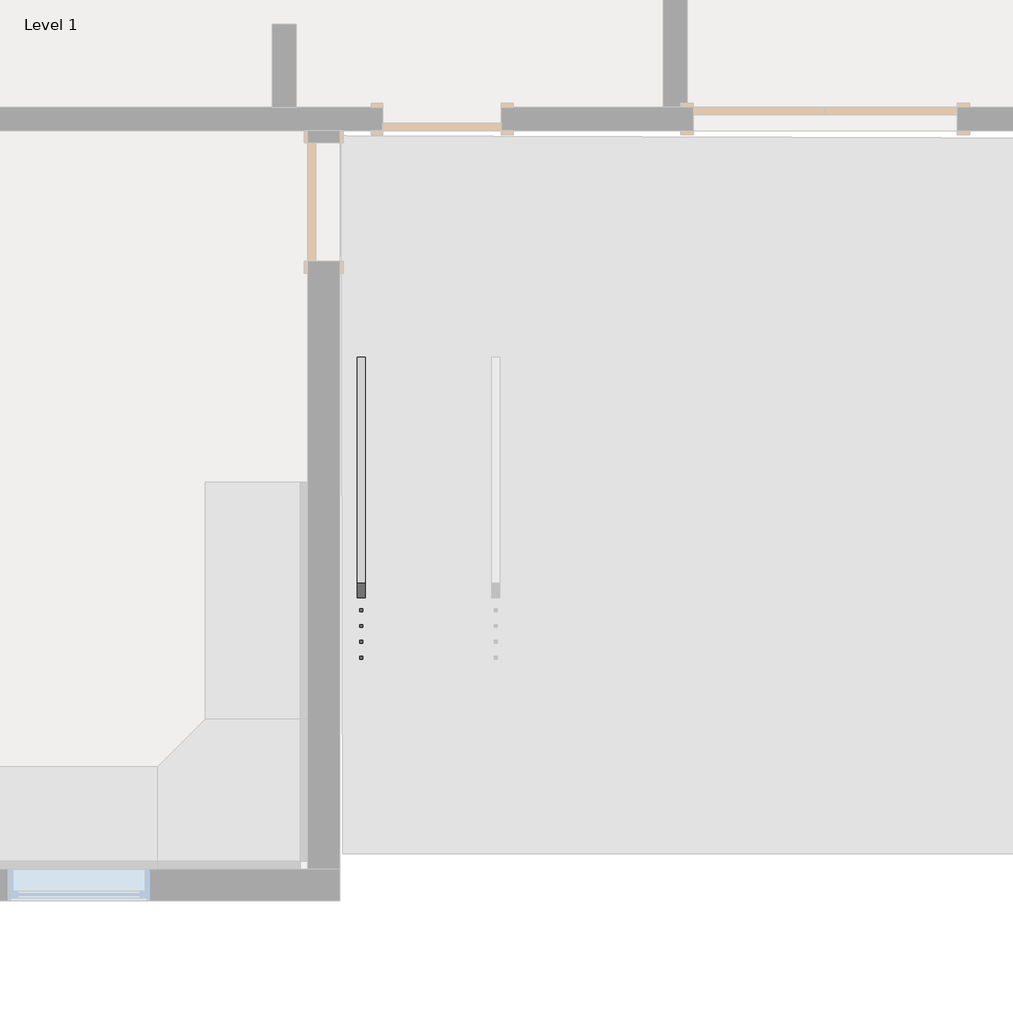
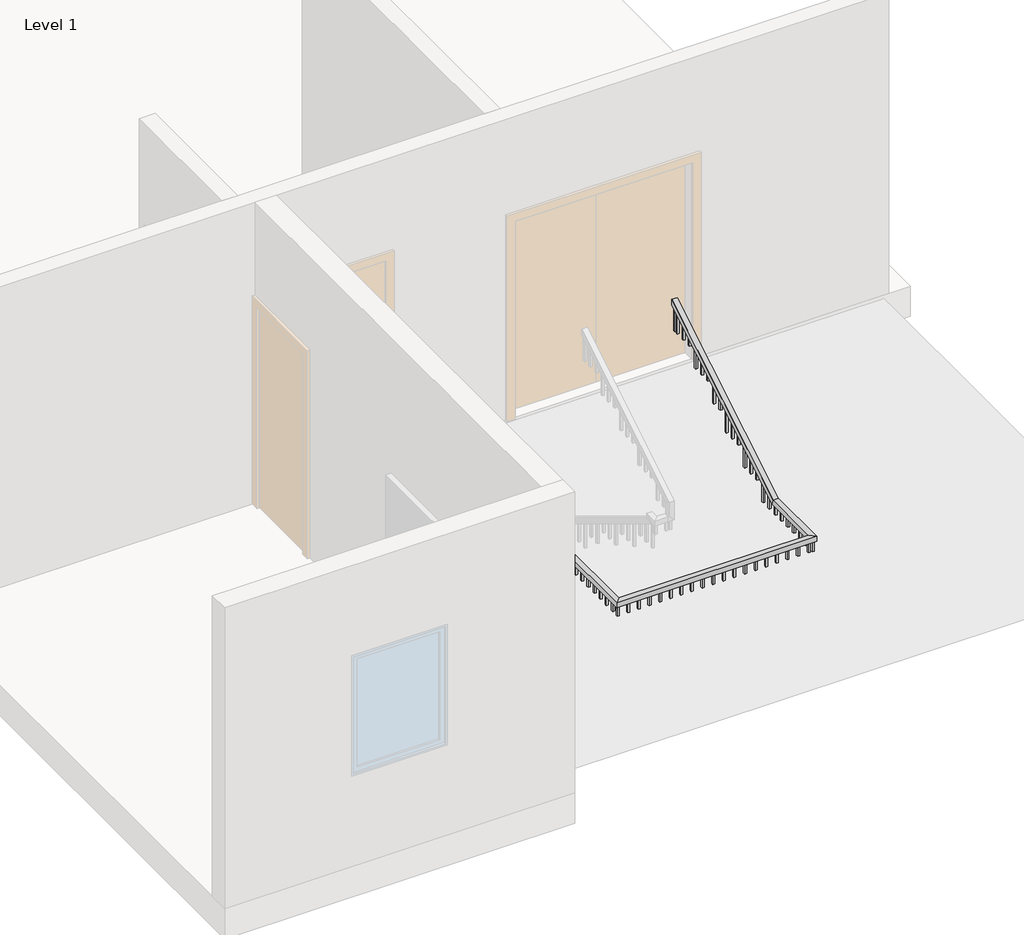
# One storey, part 2 of 3: 1 railing.
"""IFC4 building model written with IfcOpenShell, lengths in millimetres."""

from ifc_helpers import new_model, si_unit, frame, origin, place, context, project, spatial, polyline, outline, extrude, faceted_brep, element, save

model = new_model("IFC4")

# Units and contexts
model_context = context("Model", 3, world=origin())
ifc_project = project(units=[si_unit("LENGTHUNIT", "METRE", prefix="MILLI")], contexts=[model_context])

# Site, building, storey
site = spatial("IfcSite", under=ifc_project)
building = spatial("IfcBuilding", under=site)
storey = spatial("IfcBuildingStorey", under=building, Name="Level 1", Elevation=0.0)

# Railing
placement = place(None, origin())
element("IfcRailing", 1, ObjectType="Handrail - Rectangular", at=placement, inside=storey, context=model_context, shape_type="SolidModel", body=[
    faceted_brep([(-9722.6101729, -363.6715372, 321.7333333), (-9722.6101729, -363.6715372, 262.3318731), (-9773.4101729, -363.6715372, 262.3318731), (-9773.4101729, -363.6715372, 321.7333333), (-9722.6101729, -3437.0715372, 2184.4), (-9722.6101729, -3451.2639466, 2133.6), (-9773.4101729, -3451.2639466, 2133.6), (-9773.4101729, -3437.0715372, 2184.4), (-9722.6101729, -4300.6715372, 2184.4), (-9722.6101729, -4300.6715372, 2133.6), (-9773.4101729, -4351.4715372, 2133.6), (-9773.4101729, -4351.4715372, 2184.4), (-7908.2798033, -4300.6715372, 2184.4), (-7908.2798033, -4300.6715372, 2133.6), (-7857.4798033, -4351.4715372, 2133.6), (-7857.4798033, -4351.4715372, 2184.4), (-7908.2798033, -3716.4715372, 2184.4), (-7908.2798033, -3702.2791277, 2133.6), (-7857.4798033, -3702.2791277, 2133.6), (-7857.4798033, -3716.4715372, 2184.4), (-7908.2798033, -2040.0715372, 3200.4), (-7857.4798033, -2040.0715372, 3200.4), (-7857.4798033, -2040.0715372, 3140.9985397), (-7908.2798033, -2040.0715372, 3140.9985397)], [[[0, 1, 2, 3]], [[1, 0, 4, 5]], [[2, 1, 5, 6]], [[3, 2, 6, 7]], [[0, 3, 7, 4]], [[5, 4, 8, 9]], [[6, 5, 9, 10]], [[7, 6, 10, 11]], [[4, 7, 11, 8]], [[9, 8, 12, 13]], [[10, 9, 13, 14]], [[11, 10, 14, 15]], [[8, 11, 15, 12]], [[13, 12, 16, 17]], [[14, 13, 17, 18]], [[15, 14, 18, 19]], [[12, 15, 19, 16]], [[20, 21, 22, 23]], [[17, 16, 20, 23]], [[18, 17, 23, 22]], [[19, 18, 22, 21]], [[16, 19, 21, 20]]]),
    extrude(outline(polyline([(-2100.3965372, 3104.4379337), (-2081.3465372, 3115.9833882), (-2081.3465372, 2878.6666667), (-2100.3965372, 2878.6666667), (-2100.3965372, 3104.4379337)])), frame((-7892.4048033, 0.0, 0.0), z_axis=(1.0, 0.0, 0.0), x_axis=(0.0, 1.0, 0.0)), (0.0, 0.0, 1.0), 19.05),
    extrude(outline(polyline([(-2201.9965372, 3042.8621761), (-2182.9465372, 3054.4076307), (-2182.9465372, 2878.6666667), (-2201.9965372, 2878.6666667), (-2201.9965372, 3042.8621761)])), frame((-7892.4048033, 0.0, 0.0), z_axis=(1.0, 0.0, 0.0), x_axis=(0.0, 1.0, 0.0)), (0.0, 0.0, 1.0), 19.05),
    extrude(outline(polyline([(-2303.5965372, 2981.2864185), (-2284.5465372, 2992.8318731), (-2284.5465372, 2878.6666667), (-2303.5965372, 2878.6666667), (-2303.5965372, 2981.2864185)])), frame((-7892.4048033, 0.0, 0.0), z_axis=(1.0, 0.0, 0.0), x_axis=(0.0, 1.0, 0.0)), (0.0, 0.0, 1.0), 19.05),
    extrude(outline(polyline([(-2405.1965372, 2919.710661), (-2386.1465372, 2931.2561155), (-2386.1465372, 2709.3333333), (-2405.1965372, 2709.3333333), (-2405.1965372, 2919.710661)])), frame((-7892.4048033, 0.0, 0.0), z_axis=(1.0, 0.0, 0.0), x_axis=(0.0, 1.0, 0.0)), (0.0, 0.0, 1.0), 19.05),
    extrude(outline(polyline([(-2506.7965372, 2858.1349034), (-2487.7465372, 2869.6803579), (-2487.7465372, 2709.3333333), (-2506.7965372, 2709.3333333), (-2506.7965372, 2858.1349034)])), frame((-7892.4048033, 0.0, 0.0), z_axis=(1.0, 0.0, 0.0), x_axis=(0.0, 1.0, 0.0)), (0.0, 0.0, 1.0), 19.05),
    extrude(outline(polyline([(-2608.3965372, 2796.5591458), (-2589.3465372, 2808.1046004), (-2589.3465372, 2709.3333333), (-2608.3965372, 2709.3333333), (-2608.3965372, 2796.5591458)])), frame((-7892.4048033, 0.0, 0.0), z_axis=(1.0, 0.0, 0.0), x_axis=(0.0, 1.0, 0.0)), (0.0, 0.0, 1.0), 19.05),
    extrude(outline(polyline([(-2709.9965372, 2734.9833882), (-2690.9465372, 2746.5288428), (-2690.9465372, 2540.0), (-2709.9965372, 2540.0), (-2709.9965372, 2734.9833882)])), frame((-7892.4048033, 0.0, 0.0), z_axis=(1.0, 0.0, 0.0), x_axis=(0.0, 1.0, 0.0)), (0.0, 0.0, 1.0), 19.05),
    extrude(outline(polyline([(-2811.5965372, 2673.4076307), (-2792.5465372, 2684.9530852), (-2792.5465372, 2540.0), (-2811.5965372, 2540.0), (-2811.5965372, 2673.4076307)])), frame((-7892.4048033, 0.0, 0.0), z_axis=(1.0, 0.0, 0.0), x_axis=(0.0, 1.0, 0.0)), (0.0, 0.0, 1.0), 19.05),
    extrude(outline(polyline([(-2913.1965372, 2611.8318731), (-2894.1465372, 2623.3773276), (-2894.1465372, 2370.6666667), (-2913.1965372, 2370.6666667), (-2913.1965372, 2611.8318731)])), frame((-7892.4048033, 0.0, 0.0), z_axis=(1.0, 0.0, 0.0), x_axis=(0.0, 1.0, 0.0)), (0.0, 0.0, 1.0), 19.05),
    extrude(outline(polyline([(-3014.7965372, 2550.2561155), (-2995.7465372, 2561.80157), (-2995.7465372, 2370.6666667), (-3014.7965372, 2370.6666667), (-3014.7965372, 2550.2561155)])), frame((-7892.4048033, 0.0, 0.0), z_axis=(1.0, 0.0, 0.0), x_axis=(0.0, 1.0, 0.0)), (0.0, 0.0, 1.0), 19.05),
    extrude(outline(polyline([(-3116.3965372, 2488.6803579), (-3097.3465372, 2500.2258125), (-3097.3465372, 2370.6666667), (-3116.3965372, 2370.6666667), (-3116.3965372, 2488.6803579)])), frame((-7892.4048033, 0.0, 0.0), z_axis=(1.0, 0.0, 0.0), x_axis=(0.0, 1.0, 0.0)), (0.0, 0.0, 1.0), 19.05),
    extrude(outline(polyline([(-3217.9965372, 2427.1046004), (-3198.9465372, 2438.6500549), (-3198.9465372, 2201.3333333), (-3217.9965372, 2201.3333333), (-3217.9965372, 2427.1046004)])), frame((-7892.4048033, 0.0, 0.0), z_axis=(1.0, 0.0, 0.0), x_axis=(0.0, 1.0, 0.0)), (0.0, 0.0, 1.0), 19.05),
    extrude(outline(polyline([(-3319.5965372, 2365.5288428), (-3300.5465372, 2377.0742973), (-3300.5465372, 2201.3333333), (-3319.5965372, 2201.3333333), (-3319.5965372, 2365.5288428)])), frame((-7892.4048033, 0.0, 0.0), z_axis=(1.0, 0.0, 0.0), x_axis=(0.0, 1.0, 0.0)), (0.0, 0.0, 1.0), 19.05),
    extrude(outline(polyline([(-3421.1965372, 2303.9530852), (-3402.1465372, 2315.4985397), (-3402.1465372, 2201.3333333), (-3421.1965372, 2201.3333333), (-3421.1965372, 2303.9530852)])), frame((-7892.4048033, 0.0, 0.0), z_axis=(1.0, 0.0, 0.0), x_axis=(0.0, 1.0, 0.0)), (0.0, 0.0, 1.0), 19.05),
    extrude(outline(polyline([(-3522.7965372, 2242.3773276), (-3503.7465372, 2253.9227822), (-3503.7465372, 2032.0), (-3522.7965372, 2032.0), (-3522.7965372, 2242.3773276)])), frame((-7892.4048033, 0.0, 0.0), z_axis=(1.0, 0.0, 0.0), x_axis=(0.0, 1.0, 0.0)), (0.0, 0.0, 1.0), 19.05),
    extrude(outline(polyline([(-3624.3965372, 2180.80157), (-3605.3465372, 2192.3470246), (-3605.3465372, 2032.0), (-3624.3965372, 2032.0), (-3624.3965372, 2180.80157)])), frame((-7892.4048033, 0.0, 0.0), z_axis=(1.0, 0.0, 0.0), x_axis=(0.0, 1.0, 0.0)), (0.0, 0.0, 1.0), 19.05),
    extrude(outline(polyline([(-7873.3548033, -3827.5965372), (-7892.4048033, -3827.5965372), (-7892.4048033, -3808.5465372), (-7873.3548033, -3808.5465372), (-7873.3548033, -3827.5965372)])), frame((0.0, 0.0, 2032.0), z_axis=(0.0, 0.0, 1.0), x_axis=(1.0, 0.0, 0.0)), (0.0, 0.0, 1.0), 101.6),
    extrude(outline(polyline([(-7873.3548033, -3929.1965372), (-7892.4048033, -3929.1965372), (-7892.4048033, -3910.1465372), (-7873.3548033, -3910.1465372), (-7873.3548033, -3929.1965372)])), frame((0.0, 0.0, 2032.0), z_axis=(0.0, 0.0, 1.0), x_axis=(1.0, 0.0, 0.0)), (0.0, 0.0, 1.0), 101.6),
    extrude(outline(polyline([(-7873.3548033, -4030.7965372), (-7892.4048033, -4030.7965372), (-7892.4048033, -4011.7465372), (-7873.3548033, -4011.7465372), (-7873.3548033, -4030.7965372)])), frame((0.0, 0.0, 2032.0), z_axis=(0.0, 0.0, 1.0), x_axis=(1.0, 0.0, 0.0)), (0.0, 0.0, 1.0), 101.6),
    extrude(outline(polyline([(-7873.3548033, -4132.3965372), (-7892.4048033, -4132.3965372), (-7892.4048033, -4113.3465372), (-7873.3548033, -4113.3465372), (-7873.3548033, -4132.3965372)])), frame((0.0, 0.0, 2032.0), z_axis=(0.0, 0.0, 1.0), x_axis=(1.0, 0.0, 0.0)), (0.0, 0.0, 1.0), 101.6),
    extrude(outline(polyline([(-7873.3548033, -4233.9965372), (-7892.4048033, -4233.9965372), (-7892.4048033, -4214.9465372), (-7873.3548033, -4214.9465372), (-7873.3548033, -4233.9965372)])), frame((0.0, 0.0, 2032.0), z_axis=(0.0, 0.0, 1.0), x_axis=(1.0, 0.0, 0.0)), (0.0, 0.0, 1.0), 101.6),
    extrude(outline(polyline([(-7928.7351729, -4335.5965372), (-7928.7351729, -4316.5465372), (-7909.6851729, -4316.5465372), (-7909.6851729, -4335.5965372), (-7928.7351729, -4335.5965372)])), frame((0.0, 0.0, 2032.0), z_axis=(0.0, 0.0, 1.0), x_axis=(1.0, 0.0, 0.0)), (0.0, 0.0, 1.0), 101.6),
    extrude(outline(polyline([(-8030.3351729, -4335.5965372), (-8030.3351729, -4316.5465372), (-8011.2851729, -4316.5465372), (-8011.2851729, -4335.5965372), (-8030.3351729, -4335.5965372)])), frame((0.0, 0.0, 2032.0), z_axis=(0.0, 0.0, 1.0), x_axis=(1.0, 0.0, 0.0)), (0.0, 0.0, 1.0), 101.6),
    extrude(outline(polyline([(-8131.9351729, -4335.5965372), (-8131.9351729, -4316.5465372), (-8112.8851729, -4316.5465372), (-8112.8851729, -4335.5965372), (-8131.9351729, -4335.5965372)])), frame((0.0, 0.0, 2032.0), z_axis=(0.0, 0.0, 1.0), x_axis=(1.0, 0.0, 0.0)), (0.0, 0.0, 1.0), 101.6),
    extrude(outline(polyline([(-8233.5351729, -4335.5965372), (-8233.5351729, -4316.5465372), (-8214.4851729, -4316.5465372), (-8214.4851729, -4335.5965372), (-8233.5351729, -4335.5965372)])), frame((0.0, 0.0, 2032.0), z_axis=(0.0, 0.0, 1.0), x_axis=(1.0, 0.0, 0.0)), (0.0, 0.0, 1.0), 101.6),
    extrude(outline(polyline([(-8335.1351729, -4335.5965372), (-8335.1351729, -4316.5465372), (-8316.0851729, -4316.5465372), (-8316.0851729, -4335.5965372), (-8335.1351729, -4335.5965372)])), frame((0.0, 0.0, 2032.0), z_axis=(0.0, 0.0, 1.0), x_axis=(1.0, 0.0, 0.0)), (0.0, 0.0, 1.0), 101.6),
    extrude(outline(polyline([(-8436.7351729, -4335.5965372), (-8436.7351729, -4316.5465372), (-8417.6851729, -4316.5465372), (-8417.6851729, -4335.5965372), (-8436.7351729, -4335.5965372)])), frame((0.0, 0.0, 2032.0), z_axis=(0.0, 0.0, 1.0), x_axis=(1.0, 0.0, 0.0)), (0.0, 0.0, 1.0), 101.6),
    extrude(outline(polyline([(-8538.3351729, -4335.5965372), (-8538.3351729, -4316.5465372), (-8519.2851729, -4316.5465372), (-8519.2851729, -4335.5965372), (-8538.3351729, -4335.5965372)])), frame((0.0, 0.0, 2032.0), z_axis=(0.0, 0.0, 1.0), x_axis=(1.0, 0.0, 0.0)), (0.0, 0.0, 1.0), 101.6),
    extrude(outline(polyline([(-8639.9351729, -4335.5965372), (-8639.9351729, -4316.5465372), (-8620.8851729, -4316.5465372), (-8620.8851729, -4335.5965372), (-8639.9351729, -4335.5965372)])), frame((0.0, 0.0, 2032.0), z_axis=(0.0, 0.0, 1.0), x_axis=(1.0, 0.0, 0.0)), (0.0, 0.0, 1.0), 101.6),
    extrude(outline(polyline([(-8741.5351729, -4335.5965372), (-8741.5351729, -4316.5465372), (-8722.4851729, -4316.5465372), (-8722.4851729, -4335.5965372), (-8741.5351729, -4335.5965372)])), frame((0.0, 0.0, 2032.0), z_axis=(0.0, 0.0, 1.0), x_axis=(1.0, 0.0, 0.0)), (0.0, 0.0, 1.0), 101.6),
    extrude(outline(polyline([(-8843.1351729, -4335.5965372), (-8843.1351729, -4316.5465372), (-8824.0851729, -4316.5465372), (-8824.0851729, -4335.5965372), (-8843.1351729, -4335.5965372)])), frame((0.0, 0.0, 2032.0), z_axis=(0.0, 0.0, 1.0), x_axis=(1.0, 0.0, 0.0)), (0.0, 0.0, 1.0), 101.6),
    extrude(outline(polyline([(-8944.7351729, -4335.5965372), (-8944.7351729, -4316.5465372), (-8925.6851729, -4316.5465372), (-8925.6851729, -4335.5965372), (-8944.7351729, -4335.5965372)])), frame((0.0, 0.0, 2032.0), z_axis=(0.0, 0.0, 1.0), x_axis=(1.0, 0.0, 0.0)), (0.0, 0.0, 1.0), 101.6),
    extrude(outline(polyline([(-9046.3351729, -4335.5965372), (-9046.3351729, -4316.5465372), (-9027.2851729, -4316.5465372), (-9027.2851729, -4335.5965372), (-9046.3351729, -4335.5965372)])), frame((0.0, 0.0, 2032.0), z_axis=(0.0, 0.0, 1.0), x_axis=(1.0, 0.0, 0.0)), (0.0, 0.0, 1.0), 101.6),
    extrude(outline(polyline([(-9147.9351729, -4335.5965372), (-9147.9351729, -4316.5465372), (-9128.8851729, -4316.5465372), (-9128.8851729, -4335.5965372), (-9147.9351729, -4335.5965372)])), frame((0.0, 0.0, 2032.0), z_axis=(0.0, 0.0, 1.0), x_axis=(1.0, 0.0, 0.0)), (0.0, 0.0, 1.0), 101.6),
    extrude(outline(polyline([(-9249.5351729, -4335.5965372), (-9249.5351729, -4316.5465372), (-9230.4851729, -4316.5465372), (-9230.4851729, -4335.5965372), (-9249.5351729, -4335.5965372)])), frame((0.0, 0.0, 2032.0), z_axis=(0.0, 0.0, 1.0), x_axis=(1.0, 0.0, 0.0)), (0.0, 0.0, 1.0), 101.6),
    extrude(outline(polyline([(-9351.1351729, -4335.5965372), (-9351.1351729, -4316.5465372), (-9332.0851729, -4316.5465372), (-9332.0851729, -4335.5965372), (-9351.1351729, -4335.5965372)])), frame((0.0, 0.0, 2032.0), z_axis=(0.0, 0.0, 1.0), x_axis=(1.0, 0.0, 0.0)), (0.0, 0.0, 1.0), 101.6),
    extrude(outline(polyline([(-9452.7351729, -4335.5965372), (-9452.7351729, -4316.5465372), (-9433.6851729, -4316.5465372), (-9433.6851729, -4335.5965372), (-9452.7351729, -4335.5965372)])), frame((0.0, 0.0, 2032.0), z_axis=(0.0, 0.0, 1.0), x_axis=(1.0, 0.0, 0.0)), (0.0, 0.0, 1.0), 101.6),
    extrude(outline(polyline([(-9554.3351729, -4335.5965372), (-9554.3351729, -4316.5465372), (-9535.2851729, -4316.5465372), (-9535.2851729, -4335.5965372), (-9554.3351729, -4335.5965372)])), frame((0.0, 0.0, 2032.0), z_axis=(0.0, 0.0, 1.0), x_axis=(1.0, 0.0, 0.0)), (0.0, 0.0, 1.0), 101.6),
    extrude(outline(polyline([(-9655.9351729, -4335.5965372), (-9655.9351729, -4316.5465372), (-9636.8851729, -4316.5465372), (-9636.8851729, -4335.5965372), (-9655.9351729, -4335.5965372)])), frame((0.0, 0.0, 2032.0), z_axis=(0.0, 0.0, 1.0), x_axis=(1.0, 0.0, 0.0)), (0.0, 0.0, 1.0), 101.6),
    extrude(outline(polyline([(-9757.5351729, -4240.3465372), (-9738.4851729, -4240.3465372), (-9738.4851729, -4259.3965372), (-9757.5351729, -4259.3965372), (-9757.5351729, -4240.3465372)])), frame((0.0, 0.0, 2032.0), z_axis=(0.0, 0.0, 1.0), x_axis=(1.0, 0.0, 0.0)), (0.0, 0.0, 1.0), 101.6),
    extrude(outline(polyline([(-9757.5351729, -4138.7465372), (-9738.4851729, -4138.7465372), (-9738.4851729, -4157.7965372), (-9757.5351729, -4157.7965372), (-9757.5351729, -4138.7465372)])), frame((0.0, 0.0, 2032.0), z_axis=(0.0, 0.0, 1.0), x_axis=(1.0, 0.0, 0.0)), (0.0, 0.0, 1.0), 101.6),
    extrude(outline(polyline([(-9757.5351729, -4037.1465372), (-9738.4851729, -4037.1465372), (-9738.4851729, -4056.1965372), (-9757.5351729, -4056.1965372), (-9757.5351729, -4037.1465372)])), frame((0.0, 0.0, 2032.0), z_axis=(0.0, 0.0, 1.0), x_axis=(1.0, 0.0, 0.0)), (0.0, 0.0, 1.0), 101.6),
    extrude(outline(polyline([(-9757.5351729, -3935.5465372), (-9738.4851729, -3935.5465372), (-9738.4851729, -3954.5965372), (-9757.5351729, -3954.5965372), (-9757.5351729, -3935.5465372)])), frame((0.0, 0.0, 2032.0), z_axis=(0.0, 0.0, 1.0), x_axis=(1.0, 0.0, 0.0)), (0.0, 0.0, 1.0), 101.6),
    extrude(outline(polyline([(-9757.5351729, -3833.9465372), (-9738.4851729, -3833.9465372), (-9738.4851729, -3852.9965372), (-9757.5351729, -3852.9965372), (-9757.5351729, -3833.9465372)])), frame((0.0, 0.0, 2032.0), z_axis=(0.0, 0.0, 1.0), x_axis=(1.0, 0.0, 0.0)), (0.0, 0.0, 1.0), 101.6),
    extrude(outline(polyline([(-9757.5351729, -3732.3465372), (-9738.4851729, -3732.3465372), (-9738.4851729, -3751.3965372), (-9757.5351729, -3751.3965372), (-9757.5351729, -3732.3465372)])), frame((0.0, 0.0, 2032.0), z_axis=(0.0, 0.0, 1.0), x_axis=(1.0, 0.0, 0.0)), (0.0, 0.0, 1.0), 101.6),
    extrude(outline(polyline([(-9757.5351729, -3630.7465372), (-9738.4851729, -3630.7465372), (-9738.4851729, -3649.7965372), (-9757.5351729, -3649.7965372), (-9757.5351729, -3630.7465372)])), frame((0.0, 0.0, 2032.0), z_axis=(0.0, 0.0, 1.0), x_axis=(1.0, 0.0, 0.0)), (0.0, 0.0, 1.0), 101.6),
    extrude(outline(polyline([(-9757.5351729, -3529.1465372), (-9738.4851729, -3529.1465372), (-9738.4851729, -3548.1965372), (-9757.5351729, -3548.1965372), (-9757.5351729, -3529.1465372)])), frame((0.0, 0.0, 2032.0), z_axis=(0.0, 0.0, 1.0), x_axis=(1.0, 0.0, 0.0)), (0.0, 0.0, 1.0), 101.6),
    extrude(outline(polyline([(-3421.1965372, 2115.3773276), (-3402.1465372, 2103.8318731), (-3402.1465372, 1862.6666667), (-3421.1965372, 1862.6666667), (-3421.1965372, 2115.3773276)])), frame((-9757.5351729, 0.0, 0.0), z_axis=(1.0, 0.0, 0.0), x_axis=(0.0, 1.0, 0.0)), (0.0, 0.0, 1.0), 19.05),
    extrude(outline(polyline([(-3319.5965372, 2053.80157), (-3300.5465372, 2042.2561155), (-3300.5465372, 1862.6666667), (-3319.5965372, 1862.6666667), (-3319.5965372, 2053.80157)])), frame((-9757.5351729, 0.0, 0.0), z_axis=(1.0, 0.0, 0.0), x_axis=(0.0, 1.0, 0.0)), (0.0, 0.0, 1.0), 19.05),
    extrude(outline(polyline([(-3217.9965372, 1992.2258125), (-3198.9465372, 1980.6803579), (-3198.9465372, 1862.6666667), (-3217.9965372, 1862.6666667), (-3217.9965372, 1992.2258125)])), frame((-9757.5351729, 0.0, 0.0), z_axis=(1.0, 0.0, 0.0), x_axis=(0.0, 1.0, 0.0)), (0.0, 0.0, 1.0), 19.05),
    extrude(outline(polyline([(-3116.3965372, 1930.6500549), (-3097.3465372, 1919.1046004), (-3097.3465372, 1693.3333333), (-3116.3965372, 1693.3333333), (-3116.3965372, 1930.6500549)])), frame((-9757.5351729, 0.0, 0.0), z_axis=(1.0, 0.0, 0.0), x_axis=(0.0, 1.0, 0.0)), (0.0, 0.0, 1.0), 19.05),
    extrude(outline(polyline([(-3014.7965372, 1869.0742973), (-2995.7465372, 1857.5288428), (-2995.7465372, 1693.3333333), (-3014.7965372, 1693.3333333), (-3014.7965372, 1869.0742973)])), frame((-9757.5351729, 0.0, 0.0), z_axis=(1.0, 0.0, 0.0), x_axis=(0.0, 1.0, 0.0)), (0.0, 0.0, 1.0), 19.05),
    extrude(outline(polyline([(-2913.1965372, 1807.4985397), (-2894.1465372, 1795.9530852), (-2894.1465372, 1693.3333333), (-2913.1965372, 1693.3333333), (-2913.1965372, 1807.4985397)])), frame((-9757.5351729, 0.0, 0.0), z_axis=(1.0, 0.0, 0.0), x_axis=(0.0, 1.0, 0.0)), (0.0, 0.0, 1.0), 19.05),
    extrude(outline(polyline([(-2811.5965372, 1745.9227822), (-2792.5465372, 1734.3773276), (-2792.5465372, 1524.0), (-2811.5965372, 1524.0), (-2811.5965372, 1745.9227822)])), frame((-9757.5351729, 0.0, 0.0), z_axis=(1.0, 0.0, 0.0), x_axis=(0.0, 1.0, 0.0)), (0.0, 0.0, 1.0), 19.05),
    extrude(outline(polyline([(-2709.9965372, 1684.3470246), (-2690.9465372, 1672.80157), (-2690.9465372, 1524.0), (-2709.9965372, 1524.0), (-2709.9965372, 1684.3470246)])), frame((-9757.5351729, 0.0, 0.0), z_axis=(1.0, 0.0, 0.0), x_axis=(0.0, 1.0, 0.0)), (0.0, 0.0, 1.0), 19.05),
    extrude(outline(polyline([(-2608.3965372, 1622.771267), (-2589.3465372, 1611.2258125), (-2589.3465372, 1524.0), (-2608.3965372, 1524.0), (-2608.3965372, 1622.771267)])), frame((-9757.5351729, 0.0, 0.0), z_axis=(1.0, 0.0, 0.0), x_axis=(0.0, 1.0, 0.0)), (0.0, 0.0, 1.0), 19.05),
    extrude(outline(polyline([(-2506.7965372, 1561.1955094), (-2487.7465372, 1549.6500549), (-2487.7465372, 1354.6666667), (-2506.7965372, 1354.6666667), (-2506.7965372, 1561.1955094)])), frame((-9757.5351729, 0.0, 0.0), z_axis=(1.0, 0.0, 0.0), x_axis=(0.0, 1.0, 0.0)), (0.0, 0.0, 1.0), 19.05),
    extrude(outline(polyline([(-2405.1965372, 1499.6197519), (-2386.1465372, 1488.0742973), (-2386.1465372, 1354.6666667), (-2405.1965372, 1354.6666667), (-2405.1965372, 1499.6197519)])), frame((-9757.5351729, 0.0, 0.0), z_axis=(1.0, 0.0, 0.0), x_axis=(0.0, 1.0, 0.0)), (0.0, 0.0, 1.0), 19.05),
    extrude(outline(polyline([(-2303.5965372, 1438.0439943), (-2284.5465372, 1426.4985397), (-2284.5465372, 1185.3333333), (-2303.5965372, 1185.3333333), (-2303.5965372, 1438.0439943)])), frame((-9757.5351729, 0.0, 0.0), z_axis=(1.0, 0.0, 0.0), x_axis=(0.0, 1.0, 0.0)), (0.0, 0.0, 1.0), 19.05),
    extrude(outline(polyline([(-2201.9965372, 1376.4682367), (-2182.9465372, 1364.9227822), (-2182.9465372, 1185.3333333), (-2201.9965372, 1185.3333333), (-2201.9965372, 1376.4682367)])), frame((-9757.5351729, 0.0, 0.0), z_axis=(1.0, 0.0, 0.0), x_axis=(0.0, 1.0, 0.0)), (0.0, 0.0, 1.0), 19.05),
    extrude(outline(polyline([(-2100.3965372, 1314.8924791), (-2081.3465372, 1303.3470246), (-2081.3465372, 1185.3333333), (-2100.3965372, 1185.3333333), (-2100.3965372, 1314.8924791)])), frame((-9757.5351729, 0.0, 0.0), z_axis=(1.0, 0.0, 0.0), x_axis=(0.0, 1.0, 0.0)), (0.0, 0.0, 1.0), 19.05),
    extrude(outline(polyline([(-1998.7965372, 1253.3167216), (-1979.7465372, 1241.771267), (-1979.7465372, 1016.0), (-1998.7965372, 1016.0), (-1998.7965372, 1253.3167216)])), frame((-9757.5351729, 0.0, 0.0), z_axis=(1.0, 0.0, 0.0), x_axis=(0.0, 1.0, 0.0)), (0.0, 0.0, 1.0), 19.05),
    extrude(outline(polyline([(-1897.1965372, 1191.740964), (-1878.1465372, 1180.1955094), (-1878.1465372, 1016.0), (-1897.1965372, 1016.0), (-1897.1965372, 1191.740964)])), frame((-9757.5351729, 0.0, 0.0), z_axis=(1.0, 0.0, 0.0), x_axis=(0.0, 1.0, 0.0)), (0.0, 0.0, 1.0), 19.05),
    extrude(outline(polyline([(-1795.5965372, 1130.1652064), (-1776.5465372, 1118.6197519), (-1776.5465372, 1016.0), (-1795.5965372, 1016.0), (-1795.5965372, 1130.1652064)])), frame((-9757.5351729, 0.0, 0.0), z_axis=(1.0, 0.0, 0.0), x_axis=(0.0, 1.0, 0.0)), (0.0, 0.0, 1.0), 19.05),
    extrude(outline(polyline([(-1693.9965372, 1068.5894488), (-1674.9465372, 1057.0439943), (-1674.9465372, 846.6666667), (-1693.9965372, 846.6666667), (-1693.9965372, 1068.5894488)])), frame((-9757.5351729, 0.0, 0.0), z_axis=(1.0, 0.0, 0.0), x_axis=(0.0, 1.0, 0.0)), (0.0, 0.0, 1.0), 19.05),
    extrude(outline(polyline([(-1592.3965372, 1007.0136913), (-1573.3465372, 995.4682367), (-1573.3465372, 846.6666667), (-1592.3965372, 846.6666667), (-1592.3965372, 1007.0136913)])), frame((-9757.5351729, 0.0, 0.0), z_axis=(1.0, 0.0, 0.0), x_axis=(0.0, 1.0, 0.0)), (0.0, 0.0, 1.0), 19.05),
    extrude(outline(polyline([(-1490.7965372, 945.4379337), (-1471.7465372, 933.8924791), (-1471.7465372, 846.6666667), (-1490.7965372, 846.6666667), (-1490.7965372, 945.4379337)])), frame((-9757.5351729, 0.0, 0.0), z_axis=(1.0, 0.0, 0.0), x_axis=(0.0, 1.0, 0.0)), (0.0, 0.0, 1.0), 19.05),
    extrude(outline(polyline([(-1389.1965372, 883.8621761), (-1370.1465372, 872.3167216), (-1370.1465372, 677.3333333), (-1389.1965372, 677.3333333), (-1389.1965372, 883.8621761)])), frame((-9757.5351729, 0.0, 0.0), z_axis=(1.0, 0.0, 0.0), x_axis=(0.0, 1.0, 0.0)), (0.0, 0.0, 1.0), 19.05),
    extrude(outline(polyline([(-1287.5965372, 822.2864185), (-1268.5465372, 810.740964), (-1268.5465372, 677.3333333), (-1287.5965372, 677.3333333), (-1287.5965372, 822.2864185)])), frame((-9757.5351729, 0.0, 0.0), z_axis=(1.0, 0.0, 0.0), x_axis=(0.0, 1.0, 0.0)), (0.0, 0.0, 1.0), 19.05),
    extrude(outline(polyline([(-1185.9965372, 760.710661), (-1166.9465372, 749.1652064), (-1166.9465372, 508.0), (-1185.9965372, 508.0), (-1185.9965372, 760.710661)])), frame((-9757.5351729, 0.0, 0.0), z_axis=(1.0, 0.0, 0.0), x_axis=(0.0, 1.0, 0.0)), (0.0, 0.0, 1.0), 19.05),
    extrude(outline(polyline([(-1084.3965372, 699.1349034), (-1065.3465372, 687.5894488), (-1065.3465372, 508.0), (-1084.3965372, 508.0), (-1084.3965372, 699.1349034)])), frame((-9757.5351729, 0.0, 0.0), z_axis=(1.0, 0.0, 0.0), x_axis=(0.0, 1.0, 0.0)), (0.0, 0.0, 1.0), 19.05),
    extrude(outline(polyline([(-982.7965372, 637.5591458), (-963.7465372, 626.0136913), (-963.7465372, 508.0), (-982.7965372, 508.0), (-982.7965372, 637.5591458)])), frame((-9757.5351729, 0.0, 0.0), z_axis=(1.0, 0.0, 0.0), x_axis=(0.0, 1.0, 0.0)), (0.0, 0.0, 1.0), 19.05),
    extrude(outline(polyline([(-881.1965372, 575.9833882), (-862.1465372, 564.4379337), (-862.1465372, 338.6666667), (-881.1965372, 338.6666667), (-881.1965372, 575.9833882)])), frame((-9757.5351729, 0.0, 0.0), z_axis=(1.0, 0.0, 0.0), x_axis=(0.0, 1.0, 0.0)), (0.0, 0.0, 1.0), 19.05),
    extrude(outline(polyline([(-779.5965372, 514.4076307), (-760.5465372, 502.8621761), (-760.5465372, 338.6666667), (-779.5965372, 338.6666667), (-779.5965372, 514.4076307)])), frame((-9757.5351729, 0.0, 0.0), z_axis=(1.0, 0.0, 0.0), x_axis=(0.0, 1.0, 0.0)), (0.0, 0.0, 1.0), 19.05),
    extrude(outline(polyline([(-677.9965372, 452.8318731), (-658.9465372, 441.2864185), (-658.9465372, 338.6666667), (-677.9965372, 338.6666667), (-677.9965372, 452.8318731)])), frame((-9757.5351729, 0.0, 0.0), z_axis=(1.0, 0.0, 0.0), x_axis=(0.0, 1.0, 0.0)), (0.0, 0.0, 1.0), 19.05),
    extrude(outline(polyline([(-576.3965372, 391.2561155), (-557.3465372, 379.710661), (-557.3465372, 169.3333333), (-576.3965372, 169.3333333), (-576.3965372, 391.2561155)])), frame((-9757.5351729, 0.0, 0.0), z_axis=(1.0, 0.0, 0.0), x_axis=(0.0, 1.0, 0.0)), (0.0, 0.0, 1.0), 19.05),
    extrude(outline(polyline([(-474.7965372, 329.6803579), (-455.7465372, 318.1349034), (-455.7465372, 169.3333333), (-474.7965372, 169.3333333), (-474.7965372, 329.6803579)])), frame((-9757.5351729, 0.0, 0.0), z_axis=(1.0, 0.0, 0.0), x_axis=(0.0, 1.0, 0.0)), (0.0, 0.0, 1.0), 19.05),
    extrude(outline(polyline([(-7873.3548033, -3725.9965372), (-7892.4048033, -3725.9965372), (-7892.4048033, -3706.9465372), (-7873.3548033, -3706.9465372), (-7873.3548033, -3725.9965372)])), frame((0.0, 0.0, 2032.0), z_axis=(0.0, 0.0, 1.0), x_axis=(1.0, 0.0, 0.0)), (0.0, 0.0, 1.0), 101.6),
    extrude(outline(polyline([(-7892.4048033, -4335.5965372), (-7892.4048033, -4316.5465372), (-7873.3548033, -4316.5465372), (-7873.3548033, -4335.5965372), (-7892.4048033, -4335.5965372)])), frame((0.0, 0.0, 2032.0), z_axis=(0.0, 0.0, 1.0), x_axis=(1.0, 0.0, 0.0)), (0.0, 0.0, 1.0), 101.6),
    extrude(outline(polyline([(-9757.5351729, -4316.5465372), (-9738.4851729, -4316.5465372), (-9738.4851729, -4335.5965372), (-9757.5351729, -4335.5965372), (-9757.5351729, -4316.5465372)])), frame((0.0, 0.0, 2032.0), z_axis=(0.0, 0.0, 1.0), x_axis=(1.0, 0.0, 0.0)), (0.0, 0.0, 1.0), 101.6),
    extrude(outline(polyline([(-3446.5965372, 2130.771267), (-3427.5465372, 2119.2258125), (-3427.5465372, 2032.0), (-3446.5965372, 2032.0), (-3446.5965372, 2130.771267)])), frame((-9757.5351729, 0.0, 0.0), z_axis=(1.0, 0.0, 0.0), x_axis=(0.0, 1.0, 0.0)), (0.0, 0.0, 1.0), 19.05),
    extrude(outline(polyline([(-2059.1215372, 3129.4530852), (-2040.0715372, 3140.9985397), (-2040.0715372, 2878.6666667), (-2059.1215372, 2878.6666667), (-2059.1215372, 3129.4530852)])), frame((-7892.4048033, 0.0, 0.0), z_axis=(1.0, 0.0, 0.0), x_axis=(0.0, 1.0, 0.0)), (0.0, 0.0, 1.0), 19.05),
    extrude(outline(polyline([(-382.7215372, 273.8773276), (-363.6715372, 262.3318731), (-363.6715372, 169.3333333), (-382.7215372, 169.3333333), (-382.7215372, 273.8773276)])), frame((-9757.5351729, 0.0, 0.0), z_axis=(1.0, 0.0, 0.0), x_axis=(0.0, 1.0, 0.0)), (0.0, 0.0, 1.0), 19.05),
])

save(model, "model.ifc")

# Revit data of these elements
# Type "Handrail - Rectangular"
#   Assembly Code = "C2010400"
#   built-in parameter 1008612 = 0.0416667 (stored number, unit not read)
#   built-in parameter 1008611 = 0.0416667 (stored number, unit not read)
#   built-in parameter 1008609 = 0.333333 (stored number, unit not read)
#   built-in parameter 1008604 = 0.166667 (stored number, unit not read)
#   built-in parameter 1008603 = 0.166667 (stored number, unit not read)
#   Railing Height = 0' - 6"
#   built-in parameter 1008630 = 2
#   built-in parameter 1008610 = 2
#   built-in parameter 1008618 = Baluster - Square : 3/4"
# Element 1 (IfcRailing, "Handrail - Rectangular")
#   Phase Created = New Construction
